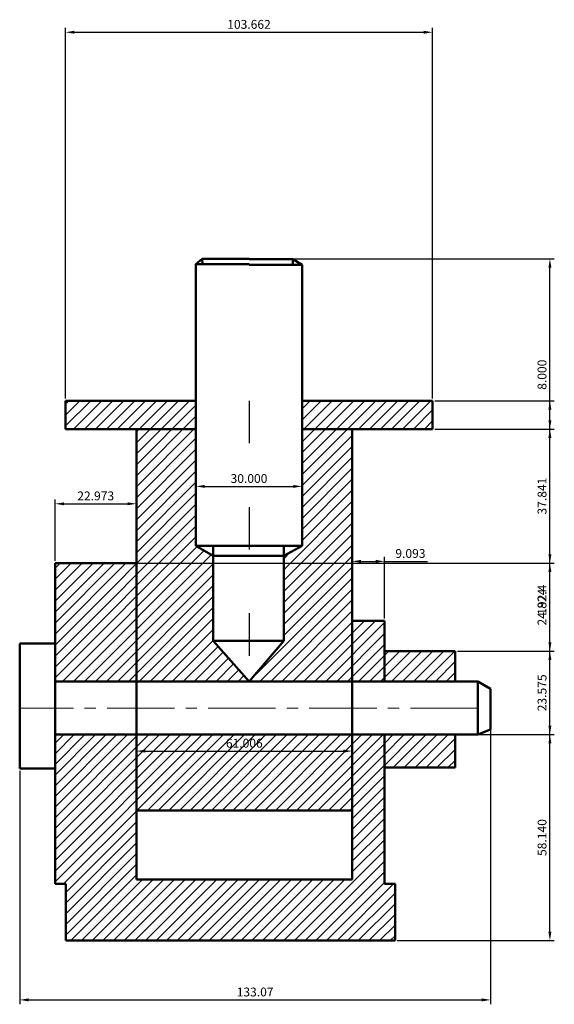
# Model space of a CAD drawing. Units: millimetres. Extents: x 1132 to 1696, y 1793 to 2376.
# Tile 4 of 4: x 1545 to 1696, y 2098 to 2376. Entities that reach past the tile are written whole.
import ezdxf

# ---------------------------------------------------------------- set-up
doc = ezdxf.new("R2010")
doc.units = ezdxf.units.MM
doc.linetypes.add('ACAD_ISO03W100', pattern=[30, 12, -18])
doc.linetypes.add('CENTER2', pattern=[28.575, 19.05, -3.175, 3.175, -3.175])
for name, color, linetype, lineweight in [('M-CNTR', 1, 'CENTER2', 18), ('M-DIMS', 2, 'Continuous', 25), ('M-HATC', 8, 'Continuous', 18), ('M-HIDN', 3, 'ACAD_ISO03W100', 25), ('M-OUTL', 7, 'Continuous', 50)]:
    doc.layers.add(name, color=color, linetype=linetype, lineweight=lineweight)
doc.styles.get("Standard").update_dxf_attribs({"font": 'arial.ttf'})
doc.dimstyles.new('ISO-25', dxfattribs={"dimtxt": 2.5, "dimasz": 2.5, "dimexe": 1.25, "dimexo": 0.625, "dimtad": 1, "dimtxsty": 'Standard', "dimcen": 2.5, "dimadec": 0, "dimazin": 0, "dimtfac": 1, "dimtmove": 0, "dimatfit": 3, "dimfxl": 1, "dimarcsym": 0})

# ---------------------------------------------------------------- blocks, each defined once
blk = doc.blocks.new('*D37')
at = {"layer": 'Defpoints', "color": 0, "transparency": 16777216}
for p in [(1677.92, 2186.94), (1544.85, 2164.4), (1677.92, 2099.11)]:
    blk.add_point(p, dxfattribs=at)
at = {"layer": 'M-DIMS', "color": 0, "lineweight": -2, "transparency": 16777216}
for p, q in [((1677.92, 2186.32), (1677.92, 2097.86)), ((1544.85, 2163.77), (1544.85, 2097.86)), ((1547.35, 2099.11), (1675.42, 2099.11))]:
    blk.add_line(p, q, dxfattribs=at)
at = {"layer": 'M-DIMS', "color": 0, "transparency": 16777216}
for points in [[(1547.35, 2099.53), (1547.35, 2098.69), (1544.85, 2099.11)], [(1675.42, 2099.53), (1675.42, 2098.69), (1677.92, 2099.11)]]:
    blk.add_solid(points, dxfattribs=at)
at = {"layer": 'M-DIMS', "color": 0, "transparency": 16777216, "insert": (1611.38, 2101.01), "char_height": 2.5, "attachment_point": 5}
blk.add_mtext('133.07', dxfattribs=at)
blk = doc.blocks.new('*D38')
at = {"layer": 'Defpoints', "color": 0, "transparency": 16777216}
for p in [(1596.44, 2308.28), (1694.67, 2308.28), (1650.92, 2115.86)]:
    blk.add_point(p, dxfattribs=at)
at = {"layer": 'M-DIMS', "color": 0, "lineweight": -2, "transparency": 16777216}
for p, q in [((1597.07, 2308.28), (1695.92, 2308.28)), ((1694.67, 2118.36), (1694.67, 2305.78)), ((1651.55, 2115.86), (1695.92, 2115.86))]:
    blk.add_line(p, q, dxfattribs=at)
at = {"layer": 'M-DIMS', "color": 0, "transparency": 16777216}
for points in [[(1694.25, 2305.78), (1695.09, 2305.78), (1694.67, 2308.28)], [(1694.25, 2118.36), (1695.09, 2118.36), (1694.67, 2115.86)]]:
    blk.add_solid(points, dxfattribs=at)
at = {"layer": 'M-DIMS', "color": 0, "transparency": 16777216, "insert": (1692.77, 2212.07), "char_height": 2.5, "attachment_point": 5, "rotation": 90}
blk.add_mtext('192.4', dxfattribs=at)
blk = doc.blocks.new('*D68')
at = {"layer": 'Defpoints', "color": 0, "transparency": 16777216}
for p in [(1667.92, 2174), (1694.67, 2174), (1650.92, 2115.86)]:
    blk.add_point(p, dxfattribs=at)
at = {"layer": 'M-DIMS', "color": 0, "lineweight": -2, "transparency": 16777216}
for p, q in [((1668.55, 2174), (1695.92, 2174)), ((1694.67, 2118.36), (1694.67, 2171.5)), ((1651.55, 2115.86), (1695.92, 2115.86))]:
    blk.add_line(p, q, dxfattribs=at)
at = {"layer": 'M-DIMS', "color": 0, "transparency": 16777216}
for points in [[(1694.25, 2171.5), (1695.09, 2171.5), (1694.67, 2174)], [(1694.25, 2118.36), (1695.09, 2118.36), (1694.67, 2115.86)]]:
    blk.add_solid(points, dxfattribs=at)
at = {"layer": 'M-DIMS', "color": 0, "transparency": 16777216, "insert": (1692.77, 2144.93), "char_height": 2.5, "attachment_point": 5, "rotation": 90}
blk.add_mtext('58.140', dxfattribs=at)
blk = doc.blocks.new('*D69')
at = {"layer": 'Defpoints', "color": 0, "transparency": 16777216}
for p in [(1667.92, 2197.57), (1694.67, 2197.57), (1667.92, 2174)]:
    blk.add_point(p, dxfattribs=at)
at = {"layer": 'M-DIMS', "color": 0, "lineweight": -2, "transparency": 16777216}
for p, q in [((1668.55, 2197.57), (1695.92, 2197.57)), ((1694.67, 2176.5), (1694.67, 2195.07)), ((1668.55, 2174), (1695.92, 2174))]:
    blk.add_line(p, q, dxfattribs=at)
at = {"layer": 'M-DIMS', "color": 0, "transparency": 16777216}
for points in [[(1694.25, 2195.07), (1695.09, 2195.07), (1694.67, 2197.57)], [(1694.25, 2176.5), (1695.09, 2176.5), (1694.67, 2174)]]:
    blk.add_solid(points, dxfattribs=at)
at = {"layer": 'M-DIMS', "color": 0, "transparency": 16777216, "insert": (1692.77, 2185.79), "char_height": 2.5, "attachment_point": 5, "rotation": 90}
blk.add_mtext('23.575', dxfattribs=at)
blk = doc.blocks.new('*D70')
at = {"layer": 'Defpoints', "color": 0, "transparency": 16777216}
for p in [(1554.85, 2222.4), (1694.67, 2222.4), (1667.92, 2197.57)]:
    blk.add_point(p, dxfattribs=at)
at = {"layer": 'M-DIMS', "color": 0, "lineweight": -2, "transparency": 16777216}
for p, q in [((1555.47, 2222.4), (1695.92, 2222.4)), ((1694.67, 2200.07), (1694.67, 2219.9)), ((1668.55, 2197.57), (1695.92, 2197.57))]:
    blk.add_line(p, q, dxfattribs=at)
at = {"layer": 'M-DIMS', "color": 0, "transparency": 16777216}
for points in [[(1694.25, 2219.9), (1695.09, 2219.9), (1694.67, 2222.4)], [(1694.25, 2200.07), (1695.09, 2200.07), (1694.67, 2197.57)]]:
    blk.add_solid(points, dxfattribs=at)
at = {"layer": 'M-DIMS', "color": 0, "transparency": 16777216, "insert": (1692.77, 2209.99), "char_height": 2.5, "attachment_point": 5, "rotation": 90}
blk.add_mtext('24.824', dxfattribs=at)
blk = doc.blocks.new('*D71')
at = {"layer": 'Defpoints', "color": 0, "transparency": 16777216}
for p in [(1661.48, 2260.24), (1694.67, 2260.24), (1554.85, 2222.4)]:
    blk.add_point(p, dxfattribs=at)
at = {"layer": 'M-DIMS', "color": 0, "lineweight": -2, "transparency": 16777216}
for p, q in [((1662.11, 2260.24), (1695.92, 2260.24)), ((1694.67, 2224.9), (1694.67, 2257.74)), ((1555.47, 2222.4), (1695.92, 2222.4))]:
    blk.add_line(p, q, dxfattribs=at)
at = {"layer": 'M-DIMS', "color": 0, "transparency": 16777216}
for points in [[(1694.25, 2257.74), (1695.09, 2257.74), (1694.67, 2260.24)], [(1694.25, 2224.9), (1695.09, 2224.9), (1694.67, 2222.4)]]:
    blk.add_solid(points, dxfattribs=at)
at = {"layer": 'M-DIMS', "color": 0, "transparency": 16777216, "insert": (1692.77, 2241.32), "char_height": 2.5, "attachment_point": 5, "rotation": 90}
blk.add_mtext('37.841', dxfattribs=at)
blk = doc.blocks.new('*D72')
at = {"layer": 'Defpoints', "color": 0, "transparency": 16777216}
for p in [(1661.48, 2268.24), (1694.67, 2268.24), (1661.48, 2260.24)]:
    blk.add_point(p, dxfattribs=at)
at = {"layer": 'M-DIMS', "color": 0, "lineweight": -2, "transparency": 16777216}
for p, q in [((1694.67, 2268.24), (1694.67, 2280.42)), ((1662.11, 2268.24), (1695.92, 2268.24)), ((1694.67, 2262.74), (1694.67, 2265.74)), ((1662.11, 2260.24), (1695.92, 2260.24))]:
    blk.add_line(p, q, dxfattribs=at)
at = {"layer": 'M-DIMS', "color": 0, "transparency": 16777216}
for points in [[(1694.25, 2265.74), (1695.09, 2265.74), (1694.67, 2268.24)], [(1694.25, 2262.74), (1695.09, 2262.74), (1694.67, 2260.24)]]:
    blk.add_solid(points, dxfattribs=at)
at = {"layer": 'M-DIMS', "color": 0, "transparency": 16777216, "insert": (1692.77, 2275.58), "char_height": 2.5, "attachment_point": 5, "rotation": 90}
blk.add_mtext('8.000', dxfattribs=at)
blk = doc.blocks.new('*D73')
at = {"layer": 'Defpoints', "color": 0, "transparency": 16777216}
for p in [(1661.48, 2372.26), (1557.82, 2268.24), (1661.48, 2268.24)]:
    blk.add_point(p, dxfattribs=at)
at = {"layer": 'M-DIMS', "color": 0, "lineweight": -2, "transparency": 16777216}
for p, q in [((1557.82, 2268.86), (1557.82, 2373.51)), ((1560.32, 2372.26), (1658.98, 2372.26)), ((1661.48, 2268.86), (1661.48, 2373.51))]:
    blk.add_line(p, q, dxfattribs=at)
at = {"layer": 'M-DIMS', "color": 0, "transparency": 16777216}
for points in [[(1560.32, 2372.68), (1560.32, 2371.84), (1557.82, 2372.26)], [(1658.98, 2372.68), (1658.98, 2371.84), (1661.48, 2372.26)]]:
    blk.add_solid(points, dxfattribs=at)
at = {"layer": 'M-DIMS', "color": 0, "transparency": 16777216, "insert": (1609.65, 2374.16), "char_height": 2.5, "attachment_point": 5}
blk.add_mtext('103.662', dxfattribs=at)
blk = doc.blocks.new('*D74')
at = {"layer": 'Defpoints', "color": 0, "transparency": 16777216}
for p in [(1624.65, 2244.06), (1594.65, 2227.31), (1624.65, 2227.31)]:
    blk.add_point(p, dxfattribs=at)
at = {"layer": 'M-DIMS', "color": 0, "lineweight": -2, "transparency": 16777216}
for p, q in [((1594.65, 2227.93), (1594.65, 2245.31)), ((1597.15, 2244.06), (1622.15, 2244.06)), ((1624.65, 2227.93), (1624.65, 2245.31))]:
    blk.add_line(p, q, dxfattribs=at)
at = {"layer": 'M-DIMS', "color": 0, "transparency": 16777216}
for points in [[(1597.15, 2244.47), (1597.15, 2243.64), (1594.65, 2244.06)], [(1622.15, 2244.47), (1622.15, 2243.64), (1624.65, 2244.06)]]:
    blk.add_solid(points, dxfattribs=at)
at = {"layer": 'M-DIMS', "color": 0, "transparency": 16777216, "insert": (1609.65, 2245.96), "char_height": 2.5, "attachment_point": 5}
blk.add_mtext('30.000', dxfattribs=at)
blk = doc.blocks.new('*D75')
at = {"layer": 'Defpoints', "color": 0, "transparency": 16777216}
for p in [(1577.82, 2239.15), (1554.85, 2222.4), (1577.82, 2222.4)]:
    blk.add_point(p, dxfattribs=at)
at = {"layer": 'M-DIMS', "color": 0, "lineweight": -2, "transparency": 16777216}
for p, q in [((1554.85, 2223.02), (1554.85, 2240.4)), ((1577.82, 2223.02), (1577.82, 2240.4)), ((1557.35, 2239.15), (1575.32, 2239.15))]:
    blk.add_line(p, q, dxfattribs=at)
at = {"layer": 'M-DIMS', "color": 0, "transparency": 16777216}
for points in [[(1557.35, 2239.56), (1557.35, 2238.73), (1554.85, 2239.15)], [(1575.32, 2239.56), (1575.32, 2238.73), (1577.82, 2239.15)]]:
    blk.add_solid(points, dxfattribs=at)
at = {"layer": 'M-DIMS', "color": 0, "transparency": 16777216, "insert": (1566.33, 2241.05), "char_height": 2.5, "attachment_point": 5}
blk.add_mtext('22.973', dxfattribs=at)
blk = doc.blocks.new('*D76')
at = {"layer": 'Defpoints', "color": 0, "transparency": 16777216}
for p in [(1638.83, 2169.34), (1577.82, 2152.59), (1638.83, 2152.59)]:
    blk.add_point(p, dxfattribs=at)
at = {"layer": 'M-DIMS', "color": 0, "lineweight": -2, "transparency": 16777216}
for p, q in [((1577.82, 2153.21), (1577.82, 2170.59)), ((1580.32, 2169.34), (1636.33, 2169.34)), ((1638.83, 2153.21), (1638.83, 2170.59))]:
    blk.add_line(p, q, dxfattribs=at)
at = {"layer": 'M-DIMS', "color": 0, "transparency": 16777216}
for points in [[(1580.32, 2169.75), (1580.32, 2168.92), (1577.82, 2169.34)], [(1636.33, 2169.75), (1636.33, 2168.92), (1638.83, 2169.34)]]:
    blk.add_solid(points, dxfattribs=at)
at = {"layer": 'M-DIMS', "color": 0, "transparency": 16777216, "insert": (1608.32, 2171.24), "char_height": 2.5, "attachment_point": 5}
blk.add_mtext('61.006', dxfattribs=at)
blk = doc.blocks.new('*D77')
at = {"layer": 'Defpoints', "color": 0, "transparency": 16777216}
for p in [(1647.92, 2222.9), (1638.83, 2206.15), (1647.92, 2206.15)]:
    blk.add_point(p, dxfattribs=at)
at = {"layer": 'M-DIMS', "color": 0, "lineweight": -2, "transparency": 16777216}
for p, q in [((1638.83, 2206.77), (1638.83, 2224.15)), ((1647.92, 2206.77), (1647.92, 2224.15)), ((1641.33, 2222.9), (1645.42, 2222.9)), ((1647.92, 2222.9), (1660.11, 2222.9))]:
    blk.add_line(p, q, dxfattribs=at)
at = {"layer": 'M-DIMS', "color": 0, "transparency": 16777216}
for points in [[(1641.33, 2223.32), (1641.33, 2222.48), (1638.83, 2222.9)], [(1645.42, 2223.32), (1645.42, 2222.48), (1647.92, 2222.9)]]:
    blk.add_solid(points, dxfattribs=at)
at = {"layer": 'M-DIMS', "color": 0, "transparency": 16777216, "insert": (1655.26, 2224.8), "char_height": 2.5, "attachment_point": 5}
blk.add_mtext('9.093', dxfattribs=at)

msp = doc.modelspace()

# ---------------------------------------------------------------- hatches: boundary and pattern name
at = {"layer": 'M-HATC'}
h = msp.add_hatch(dxfattribs=at)
h.set_pattern_fill('ANSI31', color=256, scale=0.69)
h.paths.add_polyline_path([(1594.6525, 2268.2395), (1557.8214, 2268.2395), (1557.8214, 2260.2395), (1577.8214, 2260.2395), (1594.6525, 2260.2395)])
h.paths.add_polyline_path([(1661.4837, 2268.2395), (1624.6525, 2268.2395), (1624.6525, 2260.2395), (1638.8275, 2260.2395), (1661.4837, 2260.2395)])
h.paths.add_polyline_path([(1577.8214, 2222.3981), (1554.8483, 2222.3981), (1554.8483, 2214.3981), (1554.8483, 2188.9992), (1577.8214, 2188.9992)])
h.paths.add_polyline_path([(1599.4988, 2224.4618), (1594.6525, 2227.3057), (1594.6525, 2260.2395), (1577.8214, 2260.2395), (1577.8214, 2188.9992), (1609.6525, 2188.9992), (1599.4988, 2200.4987)])
h.paths.add_polyline_path([(1638.8275, 2260.2395), (1624.6525, 2260.2395), (1624.6525, 2227.3057), (1619.4988, 2224.4618), (1619.4988, 2200.4987), (1609.6525, 2188.9992), (1638.8275, 2188.9992)])
h.paths.add_polyline_path([(1647.9209, 2206.1487), (1638.8275, 2206.1487), (1638.8275, 2188.9992), (1647.9209, 2188.9992)])
h.paths.add_polyline_path([(1667.9209, 2197.5739), (1647.9209, 2197.5739), (1647.9209, 2188.9992), (1667.9209, 2188.9992)])
h.paths.add_polyline_path([(1667.9209, 2173.9992), (1647.9209, 2173.9992), (1647.9209, 2164.6682), (1667.9209, 2164.6682)])
h = msp.add_hatch(dxfattribs=at)
h.set_pattern_fill('ANSI31', color=256, scale=0.67)
h.paths.add_polyline_path([(1577.8214, 2173.9992), (1554.8483, 2173.9992), (1554.8483, 2131.8589), (1557.8483, 2131.8589), (1557.8483, 2115.8589), (1650.9209, 2115.8589), (1650.9209, 2131.8589), (1647.9209, 2131.8589), (1647.9209, 2173.9992), (1638.8275, 2173.9992), (1638.8275, 2133.0821), (1577.8214, 2133.0821)])
h.paths.add_polyline_path([(1638.8275, 2173.9992), (1577.8214, 2173.9992), (1577.8214, 2152.5868), (1638.8275, 2152.5868)], flags=17)

# ---------------------------------------------------------------- linework, layer by layer
at = {"layer": 'M-CNTR'}
msp.add_line((1674.3166, 2181.4992), (1544.8483, 2181.4992), dxfattribs=at)
at = {"layer": 'M-HIDN'}
for p, q in [((1609.6525, 2306.6363), (1609.6525, 2306.8186)), ((1609.6525, 2268.2395), (1609.6525, 2188.9992))]:
    msp.add_line(p, q, dxfattribs=at)
at = {"layer": 'M-OUTL'}
for p, q in [((1596.441, 2308.276), (1594.6525, 2306.8186)), ((1609.6525, 2308.276), (1596.441, 2308.276)), ((1596.441, 2308.276), (1596.4824, 2306.8186)), ((1609.6525, 2308.2303), (1622.0611, 2308.2303)), ((1622.0611, 2308.2303), (1622.031, 2306.6363)), ((1622.0611, 2308.2303), (1624.6525, 2306.6363)), ((1609.6525, 2306.8186), (1594.6525, 2306.8186)), ((1594.6525, 2227.3057), (1594.6525, 2306.8186)), ((1609.6525, 2306.6363), (1624.6525, 2306.6363)), ((1624.6525, 2306.6363), (1624.6525, 2227.3057)), ((1557.8214, 2260.2395), (1557.8214, 2268.2395)), ((1557.8214, 2268.2395), (1594.6525, 2268.2395)), ((1624.6525, 2268.2395), (1661.4837, 2268.2395)), ((1661.4837, 2268.2395), (1661.4837, 2260.2395)), ((1577.8214, 2260.2395), (1557.8214, 2260.2395)), ((1577.8214, 2188.9992), (1577.8214, 2260.2395)), ((1577.8214, 2260.2395), (1594.6525, 2260.2395)), ((1624.6525, 2260.2395), (1638.8275, 2260.2395)), ((1638.8275, 2260.2395), (1638.8275, 2188.9992)), ((1661.4837, 2260.2395), (1638.8275, 2260.2395)), ((1624.6525, 2227.3057), (1594.6525, 2227.3057)), ((1594.6525, 2227.3057), (1599.4988, 2224.4618)), ((1599.4988, 2227.3057), (1599.4988, 2200.4987)), ((1619.4988, 2200.4987), (1619.4988, 2227.3057)), ((1619.4988, 2224.4618), (1624.6525, 2227.3057)), ((1619.4988, 2224.4618), (1599.4988, 2224.4618)), ((1554.8483, 2131.8589), (1554.8483, 2222.3981)), ((1554.8483, 2222.3981), (1577.8214, 2222.3981)), ((1554.8483, 2222.3981), (1554.8483, 2222.3981)), ((1554.8483, 2222.3981), (1554.8483, 2214.3981)), ((1647.9209, 2206.1487), (1638.8275, 2206.1487)), ((1647.9209, 2188.9992), (1647.9209, 2206.1487)), ((1544.8483, 2199.705), (1544.8483, 2164.3981)), ((1544.8483, 2199.705), (1554.8483, 2199.705)), ((1599.4988, 2200.4987), (1619.4988, 2200.4987)), ((1599.4988, 2200.4987), (1609.6525, 2188.9992)), ((1609.6525, 2188.9992), (1619.4988, 2200.4987)), ((1647.9209, 2197.5739), (1667.9209, 2197.5739)), ((1667.9209, 2197.5739), (1667.9209, 2188.9992)), ((1674.3166, 2188.9992), (1554.8483, 2188.9992)), ((1577.8214, 2188.9992), (1577.8214, 2133.0821)), ((1638.8275, 2188.9992), (1638.8275, 2133.0821)), ((1674.3166, 2173.9992), (1674.3166, 2188.9992)), ((1674.3166, 2188.9992), (1677.9209, 2186.9438)), ((1677.9209, 2175.4628), (1677.9209, 2186.9438)), ((1647.9209, 2173.9992), (1554.8483, 2173.9992)), ((1647.9209, 2131.8589), (1647.9209, 2173.9992)), ((1647.9209, 2173.9992), (1674.3166, 2173.9992)), ((1667.9209, 2173.9992), (1667.9209, 2164.6682)), ((1674.3166, 2173.9992), (1677.9209, 2175.4628)), ((1544.8483, 2164.3981), (1552.8483, 2164.3981)), ((1552.8483, 2164.3981), (1554.8483, 2164.3981)), ((1667.9209, 2164.6682), (1647.9209, 2164.6682)), ((1577.8214, 2152.5868), (1638.8275, 2152.5868)), ((1557.8483, 2131.8589), (1554.8483, 2131.8589)), ((1557.8483, 2115.8589), (1557.8483, 2131.8589)), ((1577.8214, 2133.0821), (1638.8275, 2133.0821)), ((1650.9209, 2131.8589), (1647.9209, 2131.8589)), ((1650.9209, 2115.8589), (1650.9209, 2131.8589)), ((1557.8483, 2115.8589), (1650.9209, 2115.8589))]:
    msp.add_line(p, q, dxfattribs=at)

# ---------------------------------------------------------------- dimensions: what is measured, and where the dimension line sits
at = {"layer": 'M-DIMS'}
for base, p1, p2, override, picture, middle in [((1661.4837, 2372.2614), (1557.8214, 2268.2395), (1661.4837, 2268.2395), {"dimdec": 3, "dimlfac": 1, "dimrnd": 0, "dimzin": 0, "dimdsep": 46, "dimlunit": 2}, '*D73', (1609.6525, 2374.1637)), ((1624.6525, 2244.0557), (1594.6525, 2227.3057), (1624.6525, 2227.3057), {"dimdec": 3, "dimlfac": 1, "dimrnd": 0, "dimzin": 0, "dimdsep": 46, "dimlunit": 2}, '*D74', (1609.6525, 2245.958)), ((1577.8214, 2239.1481), (1554.8483, 2222.3981), (1577.8214, 2222.3981), {"dimdec": 3, "dimlfac": 1, "dimrnd": 0, "dimzin": 0, "dimdsep": 46, "dimlunit": 2}, '*D75', (1566.3348, 2241.0504)), ((1647.9209, 2222.8987), (1638.8275, 2206.1487), (1647.9209, 2206.1487), {"dimdec": 3, "dimlfac": 1, "dimrnd": 0, "dimzin": 0, "dimdsep": 46, "dimlunit": 2}, '*D77', (1655.264, 2224.8009)), ((1677.9209, 2099.1089), (1544.8483, 2164.3981), (1677.9209, 2186.9438), {"dimdec": 2, "dimlfac": 1, "dimrnd": 0, "dimzin": 0, "dimdsep": 46, "dimlunit": 2}, '*D37', (1611.3846, 2101.0112)), ((1638.8275, 2169.3368), (1577.8214, 2152.5868), (1638.8275, 2152.5868), {"dimdec": 3, "dimlfac": 1, "dimrnd": 0, "dimzin": 0, "dimdsep": 46, "dimlunit": 2}, '*D76', (1608.3245, 2171.2382))]:
    dim = msp.add_linear_dim(base=base, p1=p1, p2=p2, dimstyle='ISO-25', override=override, dxfattribs=at)
    dim.commit()
    dim.dimension.update_dxf_attribs({"geometry": picture, "text_midpoint": middle})
for base, p1, p2, override, picture, middle in [((1694.6709, 2308.276), (1650.9209, 2115.8589), (1596.441, 2308.276), {"dimdec": 1, "dimlfac": 1, "dimrnd": 0, "dimzin": 0, "dimdsep": 46, "dimlunit": 2}, '*D38', (1692.7695, 2212.0674)), ((1694.6709, 2268.2395), (1661.4837, 2260.2395), (1661.4837, 2268.2395), {"dimdec": 3, "dimlfac": 1, "dimrnd": 0, "dimzin": 0, "dimdsep": 46, "dimlunit": 2}, '*D72', (1692.7695, 2275.5801)), ((1694.6709, 2260.2395), (1554.8483, 2222.3981), (1661.4837, 2260.2395), {"dimdec": 3, "dimlfac": 1, "dimrnd": 0, "dimzin": 0, "dimdsep": 46, "dimlunit": 2}, '*D71', (1692.7687, 2241.3188)), ((1694.6709, 2222.3981), (1667.9209, 2197.5739), (1554.8483, 2222.3981), {"dimdec": 3, "dimlfac": 1, "dimrnd": 0, "dimzin": 0, "dimdsep": 46, "dimlunit": 2}, '*D70', (1692.7695, 2209.986)), ((1694.6709, 2197.5739), (1667.9209, 2173.9992), (1667.9209, 2197.5739), {"dimdec": 3, "dimlfac": 1, "dimrnd": 0, "dimzin": 0, "dimdsep": 46, "dimlunit": 2}, '*D69', (1692.7687, 2185.7866)), ((1694.6709, 2173.9992), (1650.9209, 2115.8589), (1667.9209, 2173.9992), {"dimdec": 3, "dimlfac": 1, "dimrnd": 0, "dimzin": 0, "dimdsep": 46, "dimlunit": 2}, '*D68', (1692.7695, 2144.929))]:
    dim = msp.add_linear_dim(base=base, p1=p1, p2=p2, angle=90, dimstyle='ISO-25', override=override, dxfattribs=at)
    dim.commit()
    dim.dimension.update_dxf_attribs({"geometry": picture, "text_midpoint": middle})

doc.saveas('drawing.dxf')
